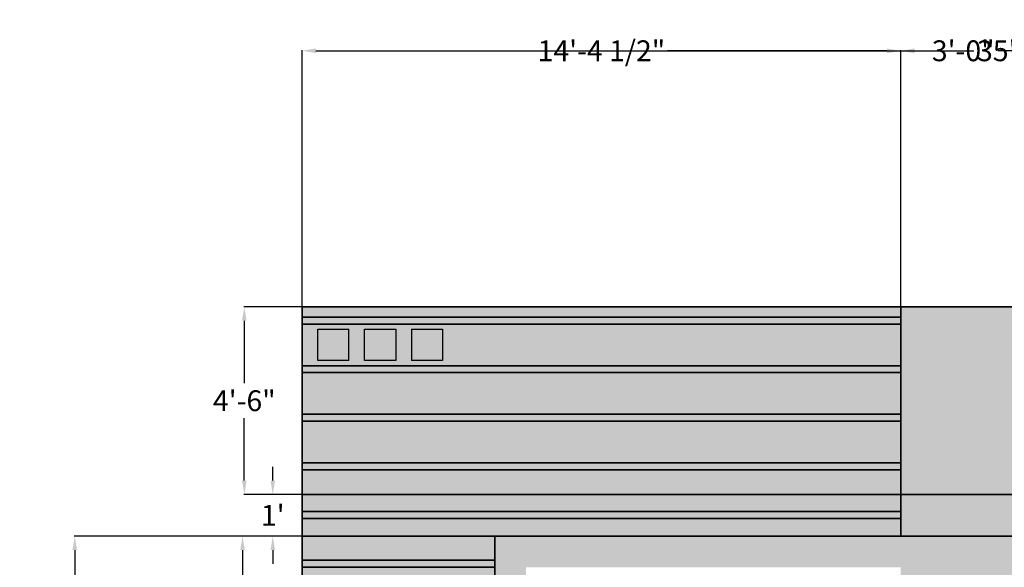
# Model space of a CAD drawing. Units: inches. Extents: x 23 to 640, y 58 to 516.
# Tile 2 of 4: x 44 to 328, y 359 to 516. Entities that reach past the tile are written whole.
import ezdxf

# ---------------------------------------------------------------- set-up
doc = ezdxf.new("R2010")
doc.units = ezdxf.units.IN
doc.header["$MEASUREMENT"] = 0
for name, color, linetype, lineweight in [('A-ANNO-DIMS', 2, 'Continuous', 18), ('A-ANNO-NPLT', 8, 'Continuous', 13), ('A-ELEV', 7, 'Continuous', 35), ('A-ELEV-PATT', 252, 'Continuous', 13), ('A-GLAZ', 4, 'Continuous', 25)]:
    doc.layers.add(name, color=color, linetype=linetype, lineweight=lineweight)
doc.styles.get("Standard").update_dxf_attribs({"font": 'arial.ttf'})
doc.dimstyles.get("Standard").update_dxf_attribs({"dimtxt": 6, "dimasz": 4, "dimexe": 0.18, "dimexo": 0.0625, "dimgap": 2, "dimtad": 0, "dimtih": 1, "dimtoh": 1, "dimdec": 0, "dimzin": 0, "dimdsep": 46, "dimlunit": 3, "dimtxsty": 'Standard', "dimcen": 2, "dimadec": 0, "dimazin": 0, "dimtfac": 1, "dimtdec": 0, "dimtofl": 0, "dimtmove": 0, "dimatfit": 3, "dimfxl": 1, "dimtolj": 1, "dimtzin": 0, "dimarcsym": 0})

# ---------------------------------------------------------------- blocks, each defined once
blk = doc.blocks.new('*D1')
at = {"layer": 'A-ANNO-DIMS', "color": 0, "lineweight": -2, "transparency": 16777216}
for p, q in [((125.37, 433.68), (108.6, 433.68)), ((108.78, 429.68), (108.78, 411.74)), ((108.78, 383.68), (108.78, 401.62)), ((125.37, 379.68), (108.6, 379.68))]:
    blk.add_line(p, q, dxfattribs=at)
at = {"layer": 'A-ANNO-DIMS', "color": 0, "transparency": 16777216}
for points in [[(108.11, 429.68), (109.44, 429.68), (108.78, 433.68)], [(108.11, 383.68), (109.44, 383.68), (108.78, 379.68)]]:
    blk.add_solid(points, dxfattribs=at)
at = {"layer": 'Defpoints', "color": 0, "transparency": 16777216}
for p in [(125.43, 433.68), (108.78, 379.68), (125.43, 379.68)]:
    blk.add_point(p, dxfattribs=at)
at = {"layer": 'A-ANNO-DIMS', "color": 0, "transparency": 16777216, "insert": (108.78, 406.68), "char_height": 6, "attachment_point": 5}
blk.add_mtext('\\A1;4\'-6"', dxfattribs=at)
blk = doc.blocks.new('*D2')
at = {"layer": 'A-ANNO-DIMS', "color": 0, "lineweight": -2, "transparency": 16777216}
for p, q in [((116.98, 383.68), (116.98, 387.68)), ((125.37, 379.68), (116.8, 379.68)), ((125.37, 367.68), (116.8, 367.68)), ((116.98, 363.68), (116.98, 359.68))]:
    blk.add_line(p, q, dxfattribs=at)
at = {"layer": 'A-ANNO-DIMS', "color": 0, "transparency": 16777216}
for points in [[(116.32, 383.68), (117.65, 383.68), (116.98, 379.68)], [(116.32, 363.68), (117.65, 363.68), (116.98, 367.68)]]:
    blk.add_solid(points, dxfattribs=at)
at = {"layer": 'Defpoints', "color": 0, "transparency": 16777216}
for p in [(125.43, 379.68), (116.98, 367.68), (125.43, 367.68)]:
    blk.add_point(p, dxfattribs=at)
at = {"layer": 'A-ANNO-DIMS', "color": 0, "transparency": 16777216, "insert": (116.98, 373.68), "char_height": 6, "attachment_point": 5}
blk.add_mtext("\\A1;1'", dxfattribs=at)
blk = doc.blocks.new('*D3')
at = {"layer": 'A-ANNO-DIMS', "color": 0, "lineweight": -2, "transparency": 16777216}
for p, q in [((125.37, 367.68), (108.09, 367.68)), ((108.27, 363.68), (108.27, 312.74)), ((108.27, 251.68), (108.27, 302.62)), ((125.37, 247.68), (108.09, 247.68))]:
    blk.add_line(p, q, dxfattribs=at)
at = {"layer": 'A-ANNO-DIMS', "color": 0, "transparency": 16777216}
for points in [[(107.61, 363.68), (108.94, 363.68), (108.27, 367.68)], [(107.61, 251.68), (108.94, 251.68), (108.27, 247.68)]]:
    blk.add_solid(points, dxfattribs=at)
at = {"layer": 'Defpoints', "color": 0, "transparency": 16777216}
for p in [(125.43, 367.68), (108.27, 247.68), (125.43, 247.68)]:
    blk.add_point(p, dxfattribs=at)
at = {"layer": 'A-ANNO-DIMS', "color": 0, "transparency": 16777216, "insert": (108.27, 307.68), "char_height": 6, "attachment_point": 5}
blk.add_mtext("\\A1;10'", dxfattribs=at)
blk = doc.blocks.new('*D17')
at = {"layer": 'A-ANNO-DIMS', "color": 0, "lineweight": -2, "transparency": 16777216}
for p, q in [((125.43, 433.74), (125.43, 507.61)), ((129.43, 507.43), (192.66, 507.43)), ((293.93, 507.43), (230.69, 507.43)), ((297.93, 433.74), (297.93, 507.61))]:
    blk.add_line(p, q, dxfattribs=at)
at = {"layer": 'A-ANNO-DIMS', "color": 0, "transparency": 16777216}
for points in [[(129.43, 508.1), (129.43, 506.76), (125.43, 507.43)], [(293.93, 508.1), (293.93, 506.76), (297.93, 507.43)]]:
    blk.add_solid(points, dxfattribs=at)
at = {"layer": 'Defpoints', "color": 0, "transparency": 16777216}
for p in [(297.93, 507.43), (125.43, 433.68), (297.93, 433.68)]:
    blk.add_point(p, dxfattribs=at)
at = {"layer": 'A-ANNO-DIMS', "color": 0, "transparency": 16777216, "insert": (211.68, 507.43), "char_height": 6, "attachment_point": 5}
blk.add_mtext('\\A1;14\'-4 1/2"', dxfattribs=at)
blk = doc.blocks.new('*D18')
at = {"layer": 'A-ANNO-DIMS', "color": 0, "lineweight": -2, "transparency": 16777216}
for p, q in [((297.93, 433.74), (297.93, 507.61)), ((301.93, 507.43), (305.96, 507.43)), ((329.93, 507.43), (325.9, 507.43)), ((333.93, 433.74), (333.93, 507.61))]:
    blk.add_line(p, q, dxfattribs=at)
at = {"layer": 'A-ANNO-DIMS', "color": 0, "transparency": 16777216}
for points in [[(301.93, 508.1), (301.93, 506.76), (297.93, 507.43)], [(329.93, 508.1), (329.93, 506.76), (333.93, 507.43)]]:
    blk.add_solid(points, dxfattribs=at)
at = {"layer": 'Defpoints', "color": 0, "transparency": 16777216}
for p in [(333.93, 507.43), (297.93, 433.68), (333.93, 433.68)]:
    blk.add_point(p, dxfattribs=at)
at = {"layer": 'A-ANNO-DIMS', "color": 0, "transparency": 16777216, "insert": (315.93, 507.43), "char_height": 6, "attachment_point": 5}
blk.add_mtext('\\A1;3\'-0"', dxfattribs=at)
blk = doc.blocks.new('*D22')
at = {"layer": 'A-ANNO-DIMS', "color": 0, "lineweight": -2, "transparency": 16777216}
for p, q in [((125.43, 433.74), (125.43, 507.61)), ((129.43, 507.43), (318.98, 507.43)), ((547.13, 507.43), (357.57, 507.43)), ((551.13, 481.74), (551.13, 507.61))]:
    blk.add_line(p, q, dxfattribs=at)
at = {"layer": 'A-ANNO-DIMS', "color": 0, "transparency": 16777216}
for points in [[(129.43, 508.1), (129.43, 506.76), (125.43, 507.43)], [(547.13, 508.1), (547.13, 506.76), (551.13, 507.43)]]:
    blk.add_solid(points, dxfattribs=at)
at = {"layer": 'Defpoints', "color": 0, "transparency": 16777216}
for p in [(551.13, 507.43), (551.13, 481.68), (125.43, 433.68)]:
    blk.add_point(p, dxfattribs=at)
at = {"layer": 'A-ANNO-DIMS', "color": 0, "transparency": 16777216, "insert": (338.28, 507.43), "char_height": 6, "attachment_point": 5}
blk.add_mtext('\\A1;35\'-5 1/2"', dxfattribs=at)
blk = doc.blocks.new('*D58')
at = {"layer": 'A-ANNO-DIMS', "color": 0, "lineweight": -2, "transparency": 16777216}
for p, q in [((297.87, 367.68), (59.75, 367.68)), ((59.93, 363.68), (59.93, 354.54)), ((59.93, 335.2), (59.93, 344.34)), ((282.87, 331.2), (59.75, 331.2))]:
    blk.add_line(p, q, dxfattribs=at)
at = {"layer": 'A-ANNO-DIMS', "color": 0, "transparency": 16777216}
for points in [[(59.26, 363.68), (60.6, 363.68), (59.93, 367.68)], [(59.26, 335.2), (60.6, 335.2), (59.93, 331.2)]]:
    blk.add_solid(points, dxfattribs=at)
at = {"layer": 'Defpoints', "color": 0, "transparency": 16777216}
for p in [(59.93, 367.68), (297.93, 367.68), (282.93, 331.2)]:
    blk.add_point(p, dxfattribs=at)
at = {"layer": 'A-ANNO-DIMS', "color": 0, "transparency": 16777216, "insert": (59.93, 349.44), "char_height": 6, "attachment_point": 5}
blk.add_mtext('\\A1;3\'-0 1/2"', dxfattribs=at)

msp = doc.modelspace()

# ---------------------------------------------------------------- hatches: boundary and pattern name
at = {"layer": 'A-ELEV-PATT'}
h = msp.add_hatch(color=256, dxfattribs=at)
h.dxf.hatch_style = 1
h.paths.add_polyline_path([(180.93, 120.76), (125.43, 120.76), (125.43, 115.68), (180.93, 115.68)])
h.paths.add_polyline_path([(180.93, 134.76), (125.43, 134.76), (125.43, 122.76), (180.93, 122.76)])
h.paths.add_polyline_path([(180.93, 148.76), (125.43, 148.76), (125.43, 136.76), (180.93, 136.76)])
h.paths.add_polyline_path([(180.93, 162.76), (125.43, 162.76), (125.43, 150.76), (180.93, 150.76)])
h.paths.add_polyline_path([(180.93, 176.76), (125.43, 176.76), (125.43, 164.76), (180.93, 164.76)])
h.paths.add_polyline_path([(180.93, 190.76), (125.43, 190.76), (125.43, 178.76), (180.93, 178.76)])
h.paths.add_polyline_path([(180.93, 204.76), (125.43, 204.76), (125.43, 192.76), (180.93, 192.76)])
h.paths.add_polyline_path([(180.93, 218.76), (125.43, 218.76), (125.43, 206.76), (180.93, 206.76)])
h.paths.add_polyline_path([(180.93, 232.76), (125.43, 232.76), (125.43, 220.76), (180.93, 220.76)])
h.paths.add_polyline_path([(180.93, 246.76), (125.43, 246.76), (125.43, 235.68), (180.93, 235.68)])
h.paths.add_polyline_path([(180.93, 235.68), (125.43, 235.68), (125.43, 234.76), (180.93, 234.76)])
h.paths.add_polyline_path([(180.93, 260.76), (125.43, 260.76), (125.43, 248.76), (180.93, 248.76)])
h.paths.add_polyline_path([(180.93, 274.76), (125.43, 274.76), (125.43, 262.76), (180.93, 262.76)])
h.paths.add_polyline_path([(180.93, 288.76), (125.43, 288.76), (125.43, 276.76), (180.93, 276.76)])
h.paths.add_polyline_path([(180.93, 302.76), (125.43, 302.76), (125.43, 290.76), (180.93, 290.76)])
h.paths.add_polyline_path([(180.93, 316.76), (125.43, 316.76), (125.43, 304.76), (180.93, 304.76)])
h.paths.add_polyline_path([(180.93, 330.76), (125.43, 330.76), (125.43, 318.76), (180.93, 318.76)])
h.paths.add_polyline_path([(180.93, 344.76), (125.43, 344.76), (125.43, 332.76), (180.93, 332.76)])
h.paths.add_polyline_path([(180.93, 358.76), (125.43, 358.76), (125.43, 346.76), (180.93, 346.76)])
h.paths.add_polyline_path([(180.93, 367.68), (125.43, 367.68), (125.43, 360.76), (180.93, 360.76)])
h.paths.add_polyline_path([(297.93, 372.76), (125.43, 372.76), (125.43, 367.68), (180.93, 367.68), (297.93, 367.68)])
h.paths.add_polyline_path([(297.93, 379.68), (125.43, 379.68), (125.43, 374.76), (297.93, 374.76)])
h.paths.add_polyline_path([(297.93, 386.76), (125.43, 386.76), (125.43, 379.68), (297.93, 379.68)])
h.paths.add_polyline_path([(297.93, 400.76), (125.43, 400.76), (125.43, 388.76), (297.93, 388.76)])
h.paths.add_polyline_path([(297.93, 414.76), (125.43, 414.76), (125.43, 402.76), (297.93, 402.76)])
h.paths.add_polyline_path([(297.93, 433.68), (125.43, 433.68), (125.43, 430.76), (297.93, 430.76)])
h.paths.add_polyline_path([(386.63, 372.76), (333.93, 372.76), (333.93, 367.68), (386.63, 367.68)])
h.paths.add_polyline_path([(386.63, 379.68), (333.93, 379.68), (333.93, 374.76), (386.63, 374.76)])
h.paths.add_polyline_path([(386.63, 386.76), (333.93, 386.76), (333.93, 379.68), (386.63, 379.68)])
h.paths.add_polyline_path([(386.63, 400.76), (333.93, 400.76), (333.93, 388.76), (386.63, 388.76)])
h.paths.add_polyline_path([(386.63, 414.76), (333.93, 414.76), (333.93, 402.76), (386.63, 402.76)])
h.paths.add_polyline_path([(386.63, 428.76), (333.93, 428.76), (333.93, 416.76), (386.63, 416.76)])
h.paths.add_polyline_path([(386.63, 433.68), (333.93, 433.68), (333.93, 430.76), (386.63, 430.76)])
h = msp.add_hatch(color=256, dxfattribs=at)
h.dxf.hatch_style = 1
h.paths.add_polyline_path([(333.93, 433.68), (297.93, 433.68), (297.93, 379.68), (333.93, 379.68)])
h.paths.add_polyline_path([(333.93, 379.68), (297.93, 379.68), (297.93, 367.68), (333.93, 367.68)])
h.paths.add_polyline_path([(333.93, 358.68), (297.93, 358.68), (297.93, 247.68), (333.93, 247.68)])
h.paths.add_polyline_path([(333.93, 229.68), (297.93, 229.68), (297.93, 215.06), (333.93, 215.06)])
h.paths.add_polyline_path([(333.93, 206.06), (297.93, 206.06), (297.93, 115.68), (333.93, 115.68)])
h = msp.add_hatch(color=256, dxfattribs=at)
h.dxf.hatch_style = 1
h.paths.add_polyline_path([(180.93, 122.76), (125.43, 122.76), (125.43, 120.76), (180.93, 120.76)])
h.paths.add_polyline_path([(180.93, 136.76), (125.43, 136.76), (125.43, 134.76), (180.93, 134.76)])
h.paths.add_polyline_path([(180.93, 150.76), (125.43, 150.76), (125.43, 148.76), (180.93, 148.76)])
h.paths.add_polyline_path([(180.93, 164.76), (125.43, 164.76), (125.43, 162.76), (180.93, 162.76)])
h.paths.add_polyline_path([(180.93, 178.76), (125.43, 178.76), (125.43, 176.76), (180.93, 176.76)])
h.paths.add_polyline_path([(180.93, 192.76), (125.43, 192.76), (125.43, 190.76), (180.93, 190.76)])
h.paths.add_polyline_path([(180.93, 206.76), (125.43, 206.76), (125.43, 204.76), (180.93, 204.76)])
h.paths.add_polyline_path([(180.93, 220.76), (125.43, 220.76), (125.43, 218.76), (180.93, 218.76)])
h.paths.add_polyline_path([(180.93, 234.76), (125.43, 234.76), (125.43, 232.76), (180.93, 232.76)])
h.paths.add_polyline_path([(180.93, 247.68), (125.43, 247.68), (125.43, 246.76), (180.93, 246.76)])
h.paths.add_polyline_path([(180.93, 248.76), (125.43, 248.76), (125.43, 247.68), (180.93, 247.68)])
h.paths.add_polyline_path([(180.93, 262.76), (125.43, 262.76), (125.43, 260.76), (180.93, 260.76)])
h.paths.add_polyline_path([(180.93, 276.76), (125.43, 276.76), (125.43, 274.76), (180.93, 274.76)])
h.paths.add_polyline_path([(180.93, 290.76), (125.43, 290.76), (125.43, 288.76), (180.93, 288.76)])
h.paths.add_polyline_path([(180.93, 304.76), (125.43, 304.76), (125.43, 302.76), (180.93, 302.76)])
h.paths.add_polyline_path([(180.93, 318.76), (125.43, 318.76), (125.43, 316.76), (180.93, 316.76)])
h.paths.add_polyline_path([(180.93, 332.76), (125.43, 332.76), (125.43, 330.76), (180.93, 330.76)])
h.paths.add_polyline_path([(180.93, 346.76), (125.43, 346.76), (125.43, 344.76), (180.93, 344.76)])
h.paths.add_polyline_path([(180.93, 360.76), (125.43, 360.76), (125.43, 358.76), (180.93, 358.76)])
h.paths.add_polyline_path([(297.93, 374.76), (125.43, 374.76), (125.43, 372.76), (297.93, 372.76)])
h.paths.add_polyline_path([(297.93, 388.76), (125.43, 388.76), (125.43, 386.76), (297.93, 386.76)])
h.paths.add_polyline_path([(297.93, 402.76), (125.43, 402.76), (125.43, 400.76), (297.93, 400.76)])
h.paths.add_polyline_path([(297.93, 416.76), (125.43, 416.76), (125.43, 414.76), (297.93, 414.76)])
h.paths.add_polyline_path([(297.93, 430.76), (125.43, 430.76), (125.43, 428.76), (297.93, 428.76)])
h.paths.add_polyline_path([(386.63, 374.76), (333.93, 374.76), (333.93, 372.76), (386.63, 372.76)])
h.paths.add_polyline_path([(386.63, 388.76), (333.93, 388.76), (333.93, 386.76), (386.63, 386.76)])
h.paths.add_polyline_path([(386.63, 402.76), (333.93, 402.76), (333.93, 400.76), (386.63, 400.76)])
h.paths.add_polyline_path([(386.63, 416.76), (333.93, 416.76), (333.93, 414.76), (386.63, 414.76)])
h.paths.add_polyline_path([(386.63, 430.76), (333.93, 430.76), (333.93, 428.76), (386.63, 428.76)])
h = msp.add_hatch(color=256, dxfattribs=at)
h.dxf.hatch_style = 1
h.paths.add_polyline_path([(297.93, 428.76), (125.43, 428.76), (125.43, 416.76), (297.93, 416.76)])
h.paths.add_polyline_path([(165.93, 418.26), (156.93, 418.26), (156.93, 427.26), (165.93, 427.26)], flags=16)
h.paths.add_polyline_path([(152.43, 418.26), (143.43, 418.26), (143.43, 427.26), (152.43, 427.26)], flags=16)
h.paths.add_polyline_path([(138.93, 418.26), (129.93, 418.26), (129.93, 427.26), (138.93, 427.26)], flags=16)
h = msp.add_hatch(color=256, dxfattribs=at)
h.dxf.hatch_style = 1
h.paths.add_polyline_path([(165.93, 427.26), (156.93, 427.26), (156.93, 418.26), (165.93, 418.26)])
h.paths.add_polyline_path([(152.43, 427.26), (143.43, 427.26), (143.43, 418.26), (152.43, 418.26)])
h.paths.add_polyline_path([(138.93, 427.26), (129.93, 427.26), (129.93, 418.26), (138.93, 418.26)])
h = msp.add_hatch(color=256, dxfattribs=at)
h.dxf.hatch_style = 1
h.paths.add_polyline_path([(371.93, 367.68), (180.93, 367.68), (180.93, 247.68), (189.93, 247.68), (189.93, 358.68), (371.93, 358.68)])
h.paths.add_polyline_path([(189.93, 247.68), (180.93, 247.68), (180.93, 235.68), (189.93, 235.68)])
h.paths.add_polyline_path([(189.93, 235.68), (180.93, 235.68), (180.93, 206.06), (333.93, 206.06), (351.93, 206.06), (351.93, 211.68), (351.93, 215.06), (189.93, 215.06)])
h.paths.add_polyline_path([(551.13, 247.68), (280.13, 247.68), (280.13, 235.68), (551.13, 235.68)])
h.paths.add_polyline_path([(551.13, 235.68), (280.13, 235.68), (280.13, 229.68), (551.13, 229.68)])

# ---------------------------------------------------------------- linework, layer by layer
at = {"layer": 'A-ANNO-NPLT'}
for p in [(125.43, 421.68), (125.43, 409.68), (125.43, 397.68), (125.43, 385.68), (125.43, 373.68), (125.43, 361.68)]:
    msp.add_point(p, dxfattribs=at)
at = {"layer": 'A-ELEV'}
for p, q in [((125.43, 115.68), (125.43, 433.68)), ((125.43, 433.68), (386.63, 433.68)), ((297.93, 433.68), (297.93, 367.68)), ((125.43, 430.76), (297.93, 430.76)), ((125.43, 428.76), (297.93, 428.76)), ((125.43, 416.76), (297.93, 416.76)), ((125.43, 414.76), (297.93, 414.76)), ((125.43, 402.76), (297.93, 402.76)), ((125.43, 400.76), (297.93, 400.76)), ((125.43, 388.76), (297.93, 388.76)), ((125.43, 386.76), (297.93, 386.76)), ((125.43, 379.68), (551.13, 379.68)), ((125.43, 374.76), (297.93, 374.76)), ((125.43, 372.76), (297.93, 372.76)), ((125.43, 367.68), (551.13, 367.68)), ((180.93, 115.68), (180.93, 367.68)), ((180.93, 367.68), (551.13, 367.68)), ((125.43, 360.76), (180.93, 360.76)), ((125.43, 358.76), (180.93, 358.76))]:
    msp.add_line(p, q, dxfattribs=at)
at = {"layer": 'A-GLAZ'}
for p, q in [((129.93, 427.26), (138.93, 427.26)), ((129.93, 418.26), (129.93, 427.26)), ((138.93, 418.26), (138.93, 427.26)), ((143.43, 418.26), (143.43, 427.26)), ((143.43, 427.26), (152.43, 427.26)), ((152.43, 427.26), (152.43, 418.26)), ((156.93, 427.26), (156.93, 418.26)), ((156.93, 427.26), (165.93, 427.26)), ((165.93, 427.26), (165.93, 418.26)), ((138.93, 418.26), (129.93, 418.26)), ((152.43, 418.26), (143.43, 418.26)), ((165.93, 418.26), (156.93, 418.26))]:
    msp.add_line(p, q, dxfattribs=at)

# ---------------------------------------------------------------- dimensions: what is measured, and where the dimension line sits
at = {"layer": 'A-ANNO-DIMS'}
for base, p1, p2, picture, middle in [((297.93, 507.43), (125.43, 433.68), (297.93, 433.68), '*D17', (211.68, 507.43)), ((551.13, 507.43), (125.43, 433.68), (551.13, 481.68), '*D22', (338.28, 507.43)), ((333.93, 507.43), (297.93, 433.68), (333.93, 433.68), '*D18', (315.93, 507.43))]:
    dim = msp.add_linear_dim(base=base, p1=p1, p2=p2, dimstyle='Standard', override={"dimdec": 1, "dimlfac": 1, "dimrnd": 0, "dimzin": 1, "dimdsep": 46, "dimlunit": 4, "dimfrac": 2}, dxfattribs=at)
    dim.commit()
    dim.dimension.update_dxf_attribs({"geometry": picture, "text_midpoint": middle})
for base, p1, p2, override, picture, middle in [((108.78, 379.68), (125.43, 433.68), (125.43, 379.68), {"dimclrd": 0, "dimclre": 0, "dimclrt": 0}, '*D1', (108.78, 406.68)), ((116.98, 367.68), (125.43, 379.68), (125.43, 367.68), {"dimclrd": 0, "dimclre": 0, "dimclrt": 0}, '*D2', (116.98, 373.68)), ((59.93, 367.68), (282.93, 331.2), (297.93, 367.68), {"dimdec": 1, "dimlfac": 1, "dimrnd": 0, "dimzin": 1, "dimdsep": 46, "dimlunit": 4, "dimfrac": 2}, '*D58', (59.93, 349.44)), ((108.27, 247.68), (125.43, 367.68), (125.43, 247.68), {"dimclrd": 0, "dimclre": 0, "dimclrt": 0}, '*D3', (108.27, 307.68))]:
    dim = msp.add_linear_dim(base=base, p1=p1, p2=p2, angle=90, dimstyle='Standard', override=override, dxfattribs=at)
    dim.commit()
    dim.dimension.update_dxf_attribs({"geometry": picture, "text_midpoint": middle})

doc.saveas('drawing.dxf')
